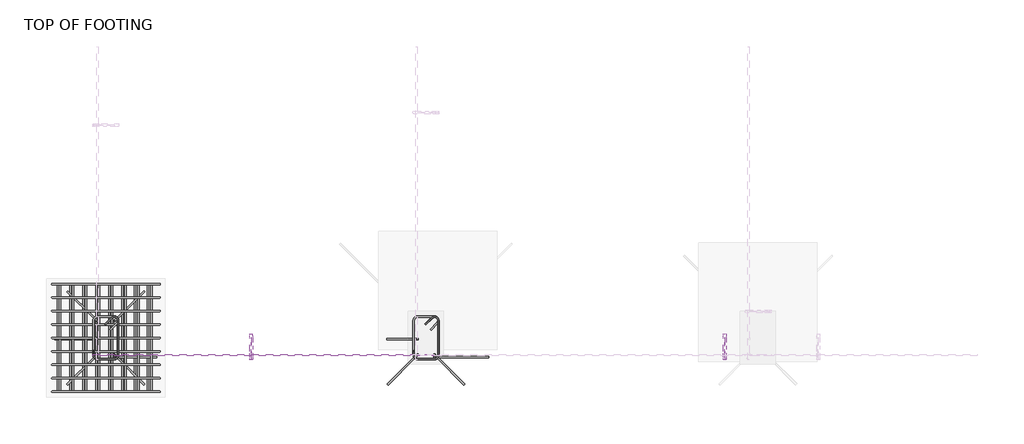
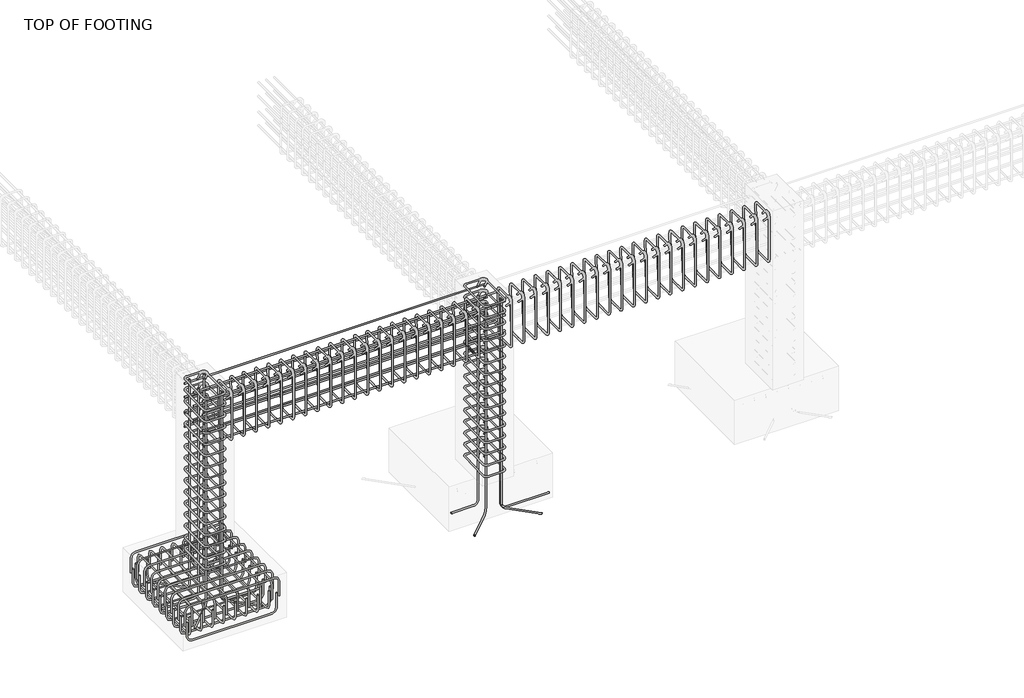
# One storey, part 2 of 14: 22 reinforcing bars.
"""IFC4 building model written with IfcOpenShell, lengths in millimetres."""

from ifc_helpers import new_model, si_unit, point, frame, origin, place, context, project, spatial, polyline, circle_curve, trimmed, segment, composite_curve, source, transform, mapped, element, save
from ifc_brep_helpers import swept_disk

model = new_model("IFC4")

# Units and contexts
model_context = context("Model", 3, world=origin())
ifc_project = project(units=[si_unit("LENGTHUNIT", "METRE", prefix="MILLI")], contexts=[model_context])

# Site, building, storey
site = spatial("IfcSite", under=ifc_project)
building = spatial("IfcBuilding", under=site)
storey = spatial("IfcBuildingStorey", under=building, Name="TOP OF FOOTING", Elevation=-1828.8)

# Reinforcing bars
placement = place(None, origin())
reinforcing_bar_shape = source(origin(), model_context, "Body", "SolidModel", [
    swept_disk(composite_curve([segment(polyline([(-3027.457813, 117.7803241, -2035.6107622), (-3027.457813, 117.7803241, -2182.9107622)]), True, "CONTINUOUS"), segment(trimmed(circle_curve(frame((-3073.807813, 117.7803241, -2182.9107622), z_axis=(0.0, 1.0, 0.0), x_axis=(46.34999999999991, 0.0, 0.0)), 46.35), [point((-3027.457813, 117.7803241, -2182.9107622))], [point((-3073.807813, 117.7803241, -2229.2607622))], True, "CARTESIAN"), True, "CONTINUOUS"), segment(polyline([(-3073.807813, 117.7803241, -2229.2607622), (-3846.4382016, 117.7803241, -2229.2607622)]), True, "CONTINUOUS"), segment(trimmed(circle_curve(frame((-3846.4382016, 117.7803241, -2182.9107622), z_axis=(0.0, 1.0, 0.0), x_axis=(0.0, 0.0, -46.34999999999991)), 46.35), [point((-3846.4382016, 117.7803241, -2229.2607622))], [point((-3892.7882016, 117.7803241, -2182.9107622))], True, "CARTESIAN"), True, "CONTINUOUS"), segment(polyline([(-3892.7882016, 117.7803241, -2182.9107622), (-3892.7882016, 117.7803241, -2035.6107622)]), True, "CONTINUOUS")], self_intersect=False), 6.35),
])
element("IfcReinforcingBar", 1, at=placement, inside=storey, context=model_context, shape_type="MappedRepresentation", body=[
    mapped(reinforcing_bar_shape, transform((0.0, 0.0, 0.0), x_axis=(1.0, 0.0, 0.0), y_axis=(0.0, 1.0, 0.0), z_axis=(0.0, 0.0, 1.0))),
    mapped(reinforcing_bar_shape, transform((0.0, -113.4125, 0.0), x_axis=(1.0, 0.0, 0.0), y_axis=(0.0, 1.0, 0.0), z_axis=(0.0, 0.0, 1.0))),
    mapped(reinforcing_bar_shape, transform((0.0, -226.825, 0.0), x_axis=(1.0, 0.0, 0.0), y_axis=(0.0, 1.0, 0.0), z_axis=(0.0, 0.0, 1.0))),
    mapped(reinforcing_bar_shape, transform((0.0, -340.2375, 0.0), x_axis=(1.0, 0.0, 0.0), y_axis=(0.0, 1.0, 0.0), z_axis=(0.0, 0.0, 1.0))),
    mapped(reinforcing_bar_shape, transform((0.0, -453.65, 0.0), x_axis=(1.0, 0.0, 0.0), y_axis=(0.0, 1.0, 0.0), z_axis=(0.0, 0.0, 1.0))),
    mapped(reinforcing_bar_shape, transform((0.0, -567.0625, 0.0), x_axis=(1.0, 0.0, 0.0), y_axis=(0.0, 1.0, 0.0), z_axis=(0.0, 0.0, 1.0))),
    mapped(reinforcing_bar_shape, transform((0.0, -680.475, 0.0), x_axis=(1.0, 0.0, 0.0), y_axis=(0.0, 1.0, 0.0), z_axis=(0.0, 0.0, 1.0))),
    mapped(reinforcing_bar_shape, transform((0.0, -793.8875, 0.0), x_axis=(1.0, 0.0, 0.0), y_axis=(0.0, 1.0, 0.0), z_axis=(0.0, 0.0, 1.0))),
    mapped(reinforcing_bar_shape, transform((0.0, -907.3, 0.0), x_axis=(1.0, 0.0, 0.0), y_axis=(0.0, 1.0, 0.0), z_axis=(0.0, 0.0, 1.0))),
])
reinforcing_bar_2_shape = source(origin(), model_context, "Body", "SolidModel", [
    swept_disk(composite_curve([segment(polyline([(-3911.0033787, 117.7803241, -2068.991024), (-3911.0033787, 117.7803241, -1921.691024)]), True, "CONTINUOUS"), segment(trimmed(circle_curve(frame((-3864.6533787, 117.7803241, -1921.691024), z_axis=(0.0, 1.0, 0.0), x_axis=(-46.350000000000364, 0.0, 0.0)), 46.35), [point((-3911.0033787, 117.7803241, -1921.691024))], [point((-3864.6533787, 117.7803241, -1875.341024))], True, "CARTESIAN"), True, "CONTINUOUS"), segment(polyline([(-3864.6533787, 117.7803241, -1875.341024), (-3050.0533787, 117.7803241, -1875.341024)]), True, "CONTINUOUS"), segment(trimmed(circle_curve(frame((-3050.0533787, 117.7803241, -1921.691024), z_axis=(0.0, 1.0, 0.0), x_axis=(0.0, 0.0, 46.34999999999991)), 46.35), [point((-3050.0533787, 117.7803241, -1875.341024))], [point((-3003.7033787, 117.7803241, -1921.691024))], True, "CARTESIAN"), True, "CONTINUOUS"), segment(polyline([(-3003.7033787, 117.7803241, -1921.691024), (-3003.7033787, 117.7803241, -2068.991024)]), True, "CONTINUOUS")], self_intersect=False), 6.35),
])
element("IfcReinforcingBar", 2, at=placement, inside=storey, context=model_context, shape_type="MappedRepresentation", body=[
    mapped(reinforcing_bar_2_shape, transform((0.0, 0.0, 0.0), x_axis=(1.0, 0.0, 0.0), y_axis=(0.0, 1.0, 0.0), z_axis=(0.0, 0.0, 1.0))),
    mapped(reinforcing_bar_2_shape, transform((0.0, -113.4125, 0.0), x_axis=(1.0, 0.0, 0.0), y_axis=(0.0, 1.0, 0.0), z_axis=(0.0, 0.0, 1.0))),
    mapped(reinforcing_bar_2_shape, transform((0.0, -226.825, 0.0), x_axis=(1.0, 0.0, 0.0), y_axis=(0.0, 1.0, 0.0), z_axis=(0.0, 0.0, 1.0))),
    mapped(reinforcing_bar_2_shape, transform((0.0, -340.2375, 0.0), x_axis=(1.0, 0.0, 0.0), y_axis=(0.0, 1.0, 0.0), z_axis=(0.0, 0.0, 1.0))),
    mapped(reinforcing_bar_2_shape, transform((0.0, -453.65, 0.0), x_axis=(1.0, 0.0, 0.0), y_axis=(0.0, 1.0, 0.0), z_axis=(0.0, 0.0, 1.0))),
    mapped(reinforcing_bar_2_shape, transform((0.0, -567.0625, 0.0), x_axis=(1.0, 0.0, 0.0), y_axis=(0.0, 1.0, 0.0), z_axis=(0.0, 0.0, 1.0))),
    mapped(reinforcing_bar_2_shape, transform((0.0, -680.475, 0.0), x_axis=(1.0, 0.0, 0.0), y_axis=(0.0, 1.0, 0.0), z_axis=(0.0, 0.0, 1.0))),
    mapped(reinforcing_bar_2_shape, transform((0.0, -793.8875, 0.0), x_axis=(1.0, 0.0, 0.0), y_axis=(0.0, 1.0, 0.0), z_axis=(0.0, 0.0, 1.0))),
    mapped(reinforcing_bar_2_shape, transform((0.0, -907.3, 0.0), x_axis=(1.0, 0.0, 0.0), y_axis=(0.0, 1.0, 0.0), z_axis=(0.0, 0.0, 1.0))),
])
reinforcing_bar_3_shape = source(origin(), model_context, "Body", "SolidModel", [
    swept_disk(composite_curve([segment(polyline([(-3073.4932847, 117.7803241, -2085.4684936), (-3073.4932847, 117.7803241, -1938.1684936)]), True, "CONTINUOUS"), segment(trimmed(circle_curve(frame((-3073.4932847, 71.4303241, -1938.1684936), z_axis=(1.0, 0.0, 0.0), x_axis=(0.0, 46.349999999999994, 0.0)), 46.35), [point((-3073.4932847, 117.7803241, -1938.1684936))], [point((-3073.4932847, 71.4303241, -1891.8184936))], True, "CARTESIAN"), True, "CONTINUOUS"), segment(polyline([(-3073.4932847, 71.4303241, -1891.8184936), (-3073.4932847, -743.1696759, -1891.8184936)]), True, "CONTINUOUS"), segment(trimmed(circle_curve(frame((-3073.4932847, -743.1696759, -1938.1684936), z_axis=(1.0, 0.0, 0.0), x_axis=(0.0, 0.0, 46.34999999999991)), 46.35), [point((-3073.4932847, -743.1696759, -1891.8184936))], [point((-3073.4932847, -789.5196759, -1938.1684936))], True, "CARTESIAN"), True, "CONTINUOUS"), segment(polyline([(-3073.4932847, -789.5196759, -1938.1684936), (-3073.4932847, -789.5196759, -2085.4684936)]), True, "CONTINUOUS")], self_intersect=False), 6.35),
])
element("IfcReinforcingBar", 3, at=placement, inside=storey, context=model_context, shape_type="MappedRepresentation", body=[
    mapped(reinforcing_bar_3_shape, transform((0.0, 0.0, 0.0), x_axis=(1.0, 0.0, 0.0), y_axis=(0.0, 1.0, 0.0), z_axis=(0.0, 0.0, 1.0))),
    mapped(reinforcing_bar_3_shape, transform((-110.0713853, 0.0, 0.0), x_axis=(1.0, 0.0, 0.0), y_axis=(0.0, 1.0, 0.0), z_axis=(0.0, 0.0, 1.0))),
    mapped(reinforcing_bar_3_shape, transform((-220.1427706, 0.0, 0.0), x_axis=(1.0, 0.0, 0.0), y_axis=(0.0, 1.0, 0.0), z_axis=(0.0, 0.0, 1.0))),
    mapped(reinforcing_bar_3_shape, transform((-330.2141558, 0.0, 0.0), x_axis=(1.0, 0.0, 0.0), y_axis=(0.0, 1.0, 0.0), z_axis=(0.0, 0.0, 1.0))),
    mapped(reinforcing_bar_3_shape, transform((-440.2855411, 0.0, 0.0), x_axis=(1.0, 0.0, 0.0), y_axis=(0.0, 1.0, 0.0), z_axis=(0.0, 0.0, 1.0))),
    mapped(reinforcing_bar_3_shape, transform((-550.3569264, 0.0, 0.0), x_axis=(1.0, 0.0, 0.0), y_axis=(0.0, 1.0, 0.0), z_axis=(0.0, 0.0, 1.0))),
    mapped(reinforcing_bar_3_shape, transform((-660.4283117, 0.0, 0.0), x_axis=(1.0, 0.0, 0.0), y_axis=(0.0, 1.0, 0.0), z_axis=(0.0, 0.0, 1.0))),
    mapped(reinforcing_bar_3_shape, transform((-770.4996969, 0.0, 0.0), x_axis=(1.0, 0.0, 0.0), y_axis=(0.0, 1.0, 0.0), z_axis=(0.0, 0.0, 1.0))),
])
reinforcing_bar_4_shape = source(origin(), model_context, "Body", "SolidModel", [
    swept_disk(composite_curve([segment(polyline([(-3862.3533787, 117.7803241, -1990.15), (-3862.3533787, 117.7803241, -2137.45)]), True, "CONTINUOUS"), segment(trimmed(circle_curve(frame((-3862.3533787, 71.4303241, -2137.45), z_axis=(-1.0, 0.0, 0.0), x_axis=(0.0, 46.349999999999994, 0.0)), 46.35), [point((-3862.3533787, 117.7803241, -2137.45))], [point((-3862.3533787, 71.4303241, -2183.8))], True, "CARTESIAN"), True, "CONTINUOUS"), segment(polyline([(-3862.3533787, 71.4303241, -2183.8), (-3862.3533787, -743.1696759, -2183.8)]), True, "CONTINUOUS"), segment(trimmed(circle_curve(frame((-3862.3533787, -743.1696759, -2137.45), z_axis=(-1.0, 0.0, 0.0), x_axis=(0.0, 0.0, -46.350000000000364)), 46.35), [point((-3862.3533787, -743.1696759, -2183.8))], [point((-3862.3533787, -789.5196759, -2137.45))], True, "CARTESIAN"), True, "CONTINUOUS"), segment(polyline([(-3862.3533787, -789.5196759, -2137.45), (-3862.3533787, -789.5196759, -1990.15)]), True, "CONTINUOUS")], self_intersect=False), 6.35),
])
element("IfcReinforcingBar", 4, at=placement, inside=storey, context=model_context, shape_type="MappedRepresentation", body=[
    mapped(reinforcing_bar_4_shape, transform((0.0, 0.0, 0.0), x_axis=(1.0, 0.0, 0.0), y_axis=(0.0, 1.0, 0.0), z_axis=(0.0, 0.0, 1.0))),
    mapped(reinforcing_bar_4_shape, transform((108.7810905, 0.0, 0.0), x_axis=(1.0, 0.0, 0.0), y_axis=(0.0, 1.0, 0.0), z_axis=(0.0, 0.0, 1.0))),
    mapped(reinforcing_bar_4_shape, transform((217.5621811, 0.0, 0.0), x_axis=(1.0, 0.0, 0.0), y_axis=(0.0, 1.0, 0.0), z_axis=(0.0, 0.0, 1.0))),
    mapped(reinforcing_bar_4_shape, transform((326.3432716, 0.0, 0.0), x_axis=(1.0, 0.0, 0.0), y_axis=(0.0, 1.0, 0.0), z_axis=(0.0, 0.0, 1.0))),
    mapped(reinforcing_bar_4_shape, transform((435.1243621, 0.0, 0.0), x_axis=(1.0, 0.0, 0.0), y_axis=(0.0, 1.0, 0.0), z_axis=(0.0, 0.0, 1.0))),
    mapped(reinforcing_bar_4_shape, transform((543.9054526, 0.0, 0.0), x_axis=(1.0, 0.0, 0.0), y_axis=(0.0, 1.0, 0.0), z_axis=(0.0, 0.0, 1.0))),
    mapped(reinforcing_bar_4_shape, transform((652.6865432, 0.0, 0.0), x_axis=(1.0, 0.0, 0.0), y_axis=(0.0, 1.0, 0.0), z_axis=(0.0, 0.0, 1.0))),
    mapped(reinforcing_bar_4_shape, transform((761.4676337, 0.0, 0.0), x_axis=(1.0, 0.0, 0.0), y_axis=(0.0, 1.0, 0.0), z_axis=(0.0, 0.0, 1.0))),
])
reinforcing_bar_5_shape = source(origin(), model_context, "Body", "SolidModel", [
    swept_disk(composite_curve([segment(polyline([(-3462.9647392, -222.1454413, -46.35), (-3407.2211763, -166.4018783, -46.35)]), True, "CONTINUOUS"), segment(trimmed(circle_curve(frame((-3385.0533787, -188.5696759, -46.35), z_axis=(0.0, 0.0, -1.0), x_axis=(-22.167797600000085, 22.1677976, 0.0)), 31.35), [point((-3407.2211763, -166.4018783, -46.35))], [point((-3353.7033787, -188.5696759, -46.35))], True, "CARTESIAN"), True, "CONTINUOUS"), segment(polyline([(-3353.7033787, -188.5696759, -46.35), (-3353.7033787, -483.1696759, -46.35)]), True, "CONTINUOUS"), segment(trimmed(circle_curve(frame((-3385.0533787, -483.1696759, -46.35), z_axis=(0.0, 0.0, -1.0), x_axis=(31.34999999999991, 0.0, 0.0)), 31.35), [point((-3353.7033787, -483.1696759, -46.35))], [point((-3385.0533787, -514.5196759, -46.35))], True, "CARTESIAN"), True, "CONTINUOUS"), segment(polyline([(-3385.0533787, -514.5196759, -46.35), (-3529.6533787, -514.5196759, -46.35)]), True, "CONTINUOUS"), segment(trimmed(circle_curve(frame((-3529.6533787, -483.189461, -45.2363875), z_axis=(0.0, 0.03552192833448213, -0.9993688971583016), x_axis=(0.0, -31.330214900000044, -1.1136125000000021)), 31.35), [point((-3529.6533787, -514.5196759, -46.35))], [point((-3561.0033787, -483.189461, -45.2363875))], True, "CARTESIAN"), True, "CONTINUOUS"), segment(polyline([(-3561.0033787, -483.189461, -45.2363875), (-3561.0033787, -188.5498908, -34.7636125)]), True, "CONTINUOUS"), segment(trimmed(circle_curve(frame((-3529.6533787, -188.5498908, -34.7636125), z_axis=(0.0, 0.03552192833448213, -0.9993688971583016), x_axis=(-31.350000000000364, 0.0, 0.0)), 31.35), [point((-3561.0033787, -188.5498908, -34.7636125))], [point((-3529.6533787, -157.2196759, -33.65))], True, "CARTESIAN"), True, "CONTINUOUS"), segment(polyline([(-3529.6533787, -157.2196759, -33.65), (-3385.0533787, -157.2196759, -33.65)]), True, "CONTINUOUS"), segment(trimmed(circle_curve(frame((-3385.0533787, -188.5696759, -33.65), z_axis=(0.0, 0.0, -1.0), x_axis=(0.0, 31.349999999999994, 0.0)), 31.35), [point((-3385.0533787, -157.2196759, -33.65))], [point((-3362.8855811, -210.7374735, -33.65))], True, "CARTESIAN"), True, "CONTINUOUS"), segment(polyline([(-3362.8855811, -210.7374735, -33.65), (-3418.6291441, -266.4810364, -33.65)]), True, "CONTINUOUS")], self_intersect=False), 6.35),
])
element("IfcReinforcingBar", 5, at=placement, inside=storey, context=model_context, shape_type="MappedRepresentation", body=[
    mapped(reinforcing_bar_5_shape, transform((0.0, 0.0, 0.0), x_axis=(1.0, 0.0, 0.0), y_axis=(0.0, 1.0, 0.0), z_axis=(0.0, 0.0, 1.0))),
    mapped(reinforcing_bar_5_shape, transform((0.0, 0.0, -115.74), x_axis=(1.0, 0.0, 0.0), y_axis=(0.0, 1.0, 0.0), z_axis=(0.0, 0.0, 1.0))),
    mapped(reinforcing_bar_5_shape, transform((0.0, 0.0, -231.48), x_axis=(1.0, 0.0, 0.0), y_axis=(0.0, 1.0, 0.0), z_axis=(0.0, 0.0, 1.0))),
    mapped(reinforcing_bar_5_shape, transform((0.0, 0.0, -347.22), x_axis=(1.0, 0.0, 0.0), y_axis=(0.0, 1.0, 0.0), z_axis=(0.0, 0.0, 1.0))),
    mapped(reinforcing_bar_5_shape, transform((0.0, 0.0, -462.96), x_axis=(1.0, 0.0, 0.0), y_axis=(0.0, 1.0, 0.0), z_axis=(0.0, 0.0, 1.0))),
    mapped(reinforcing_bar_5_shape, transform((0.0, 0.0, -578.7), x_axis=(1.0, 0.0, 0.0), y_axis=(0.0, 1.0, 0.0), z_axis=(0.0, 0.0, 1.0))),
    mapped(reinforcing_bar_5_shape, transform((0.0, 0.0, -694.44), x_axis=(1.0, 0.0, 0.0), y_axis=(0.0, 1.0, 0.0), z_axis=(0.0, 0.0, 1.0))),
    mapped(reinforcing_bar_5_shape, transform((0.0, 0.0, -810.18), x_axis=(1.0, 0.0, 0.0), y_axis=(0.0, 1.0, 0.0), z_axis=(0.0, 0.0, 1.0))),
    mapped(reinforcing_bar_5_shape, transform((0.0, 0.0, -925.92), x_axis=(1.0, 0.0, 0.0), y_axis=(0.0, 1.0, 0.0), z_axis=(0.0, 0.0, 1.0))),
    mapped(reinforcing_bar_5_shape, transform((0.0, 0.0, -1041.66), x_axis=(1.0, 0.0, 0.0), y_axis=(0.0, 1.0, 0.0), z_axis=(0.0, 0.0, 1.0))),
    mapped(reinforcing_bar_5_shape, transform((0.0, 0.0, -1157.4), x_axis=(1.0, 0.0, 0.0), y_axis=(0.0, 1.0, 0.0), z_axis=(0.0, 0.0, 1.0))),
    mapped(reinforcing_bar_5_shape, transform((0.0, 0.0, -1273.14), x_axis=(1.0, 0.0, 0.0), y_axis=(0.0, 1.0, 0.0), z_axis=(0.0, 0.0, 1.0))),
    mapped(reinforcing_bar_5_shape, transform((0.0, 0.0, -1388.88), x_axis=(1.0, 0.0, 0.0), y_axis=(0.0, 1.0, 0.0), z_axis=(0.0, 0.0, 1.0))),
    mapped(reinforcing_bar_5_shape, transform((0.0, 0.0, -1504.62), x_axis=(1.0, 0.0, 0.0), y_axis=(0.0, 1.0, 0.0), z_axis=(0.0, 0.0, 1.0))),
    mapped(reinforcing_bar_5_shape, transform((0.0, 0.0, -1620.36), x_axis=(1.0, 0.0, 0.0), y_axis=(0.0, 1.0, 0.0), z_axis=(0.0, 0.0, 1.0))),
    mapped(reinforcing_bar_5_shape, transform((0.0, 0.0, -1736.1), x_axis=(1.0, 0.0, 0.0), y_axis=(0.0, 1.0, 0.0), z_axis=(0.0, 0.0, 1.0))),
])
element("IfcReinforcingBar", 6, at=placement, inside=storey, context=model_context, shape_type="SolidModel", body=[
    swept_disk(composite_curve([segment(polyline([(-3386.7020371, -495.9487744, -40.0), (-3386.7020371, -495.9487744, -2122.4113862)]), True, "CONTINUOUS"), segment(trimmed(circle_curve(frame((-3340.3520371, -495.9487744, -2122.4113862), z_axis=(0.0, -1.0, 0.0), x_axis=(-46.34999999999991, 0.0, 0.0)), 46.35), [point((-3386.7020371, -495.9487744, -2122.4113862))], [point((-3340.3520371, -495.9487744, -2168.7613862))], True, "CARTESIAN"), True, "CONTINUOUS"), segment(polyline([(-3340.3520371, -495.9487744, -2168.7613862), (-3028.2406023, -495.9487744, -2168.7613862)]), True, "CONTINUOUS")], self_intersect=False), 6.35),
])
element("IfcReinforcingBar", 7, at=placement, inside=storey, context=model_context, shape_type="SolidModel", body=[
    swept_disk(composite_curve([segment(polyline([(-3386.7020371, -475.9487744, -40.0), (-3386.7020371, -475.9487744, -2122.4113862)]), True, "CONTINUOUS"), segment(trimmed(circle_curve(frame((-3353.9276378, -508.7231737, -2122.4113862), z_axis=(-0.7071067811865441, -0.707106781186551, 0.0), x_axis=(-32.774399299999914, 32.77439930000003, 0.0)), 46.35), [point((-3386.7020371, -475.9487744, -2122.4113862))], [point((-3353.9276378, -508.7231737, -2168.7613862))], True, "CARTESIAN"), True, "CONTINUOUS"), segment(polyline([(-3353.9276378, -508.7231737, -2168.7613862), (-3133.2315258, -729.4192858, -2168.7613862)]), True, "CONTINUOUS")], self_intersect=False), 6.35),
])
element("IfcReinforcingBar", 8, at=placement, inside=storey, context=model_context, shape_type="SolidModel", body=[
    swept_disk(composite_curve([segment(polyline([(-3528.0047203, -475.9487744, -40.0), (-3528.0047203, -475.9487744, -2122.4113862)]), True, "CONTINUOUS"), segment(trimmed(circle_curve(frame((-3560.7791196, -508.7231737, -2122.4113862), z_axis=(-0.7071067811865341, 0.707106781186561, 0.0), x_axis=(32.774399299999914, 32.77439930000003, 0.0)), 46.35), [point((-3528.0047203, -475.9487744, -2122.4113862))], [point((-3560.7791196, -508.7231737, -2168.7613862))], True, "CARTESIAN"), True, "CONTINUOUS"), segment(polyline([(-3560.7791196, -508.7231737, -2168.7613862), (-3781.4752316, -729.4192858, -2168.7613862)]), True, "CONTINUOUS")], self_intersect=False), 6.35),
])
element("IfcReinforcingBar", 9, at=placement, inside=storey, context=model_context, shape_type="SolidModel", body=[
    swept_disk(composite_curve([segment(polyline([(-3386.7020371, -195.7905774, -40.0), (-3386.7020371, -195.7905774, -2122.4113862)]), True, "CONTINUOUS"), segment(trimmed(circle_curve(frame((-3353.9276378, -163.0161781, -2122.4113862), z_axis=(0.7071067811865235, -0.7071067811865717, 0.0), x_axis=(-32.774399299999914, -32.7743993, 0.0)), 46.35), [point((-3386.7020371, -195.7905774, -2122.4113862))], [point((-3353.9276378, -163.0161781, -2168.7613862))], True, "CARTESIAN"), True, "CONTINUOUS"), segment(polyline([(-3353.9276378, -163.0161781, -2168.7613862), (-3133.2315258, 57.6799339, -2168.7613862)]), True, "CONTINUOUS")], self_intersect=False), 6.35),
])
element("IfcReinforcingBar", 10, at=placement, inside=storey, context=model_context, shape_type="SolidModel", body=[
    swept_disk(composite_curve([segment(polyline([(-3528.0047203, -195.7905774, -40.0), (-3528.0047203, -195.7905774, -2122.4113862)]), True, "CONTINUOUS"), segment(trimmed(circle_curve(frame((-3560.7791196, -163.0161781, -2122.4113862), z_axis=(0.7071067811865548, 0.7071067811865404, 0.0), x_axis=(32.774399299999914, -32.7743993, 0.0)), 46.35), [point((-3528.0047203, -195.7905774, -2122.4113862))], [point((-3560.7791196, -163.0161781, -2168.7613862))], True, "CARTESIAN"), True, "CONTINUOUS"), segment(polyline([(-3560.7791196, -163.0161781, -2168.7613862), (-3781.4752316, 57.6799339, -2168.7613862)]), True, "CONTINUOUS")], self_intersect=False), 6.35),
])
element("IfcReinforcingBar", 11, at=placement, inside=storey, context=model_context, shape_type="SolidModel", body=[
    swept_disk(composite_curve([segment(polyline([(-3528.0047203, -345.9487744, -40.0), (-3528.0047203, -345.9487744, -2122.4113862)]), True, "CONTINUOUS"), segment(trimmed(circle_curve(frame((-3574.3547203, -345.9487744, -2122.4113862), z_axis=(0.0, 1.0, 0.0), x_axis=(46.34999999999991, 0.0, 0.0)), 46.35), [point((-3528.0047203, -345.9487744, -2122.4113862))], [point((-3574.3547203, -345.9487744, -2168.7613862))], True, "CARTESIAN"), True, "CONTINUOUS"), segment(polyline([(-3574.3547203, -345.9487744, -2168.7613862), (-3886.4661551, -345.9487744, -2168.7613862)]), True, "CONTINUOUS")], self_intersect=False), 6.35),
])
reinforcing_bar_6_shape = source(origin(), model_context, "Body", "SolidModel", [
    swept_disk(composite_curve([segment(polyline([(-762.9647392, -222.1454413, -46.35), (-707.2211763, -166.4018783, -46.35)]), True, "CONTINUOUS"), segment(trimmed(circle_curve(frame((-685.0533787, -188.5696759, -46.35), z_axis=(0.0, 0.0, -1.0), x_axis=(-22.16779759999997, 22.1677976, 0.0)), 31.35), [point((-707.2211763, -166.4018783, -46.35))], [point((-653.7033787, -188.5696759, -46.35))], True, "CARTESIAN"), True, "CONTINUOUS"), segment(polyline([(-653.7033787, -188.5696759, -46.35), (-653.7033787, -483.1696759, -46.35)]), True, "CONTINUOUS"), segment(trimmed(circle_curve(frame((-685.0533787, -483.1696759, -46.35), z_axis=(0.0, 0.0, -1.0), x_axis=(31.350000000000023, 0.0, 0.0)), 31.35), [point((-653.7033787, -483.1696759, -46.35))], [point((-685.0533787, -514.5196759, -46.35))], True, "CARTESIAN"), True, "CONTINUOUS"), segment(polyline([(-685.0533787, -514.5196759, -46.35), (-829.6533787, -514.5196759, -46.35)]), True, "CONTINUOUS"), segment(trimmed(circle_curve(frame((-829.6533787, -483.189461, -45.2363875), z_axis=(0.0, 0.03552192833448213, -0.9993688971583016), x_axis=(0.0, -31.330214900000044, -1.1136125000000021)), 31.35), [point((-829.6533787, -514.5196759, -46.35))], [point((-861.0033787, -483.189461, -45.2363875))], True, "CARTESIAN"), True, "CONTINUOUS"), segment(polyline([(-861.0033787, -483.189461, -45.2363875), (-861.0033787, -188.5498908, -34.7636125)]), True, "CONTINUOUS"), segment(trimmed(circle_curve(frame((-829.6533787, -188.5498908, -34.7636125), z_axis=(0.0, 0.03552192833448213, -0.9993688971583016), x_axis=(-31.350000000000023, 0.0, 0.0)), 31.35), [point((-861.0033787, -188.5498908, -34.7636125))], [point((-829.6533787, -157.2196759, -33.65))], True, "CARTESIAN"), True, "CONTINUOUS"), segment(polyline([(-829.6533787, -157.2196759, -33.65), (-685.0533787, -157.2196759, -33.65)]), True, "CONTINUOUS"), segment(trimmed(circle_curve(frame((-685.0533787, -188.5696759, -33.65), z_axis=(0.0, 0.0, -1.0), x_axis=(0.0, 31.349999999999994, 0.0)), 31.35), [point((-685.0533787, -157.2196759, -33.65))], [point((-662.8855811, -210.7374735, -33.65))], True, "CARTESIAN"), True, "CONTINUOUS"), segment(polyline([(-662.8855811, -210.7374735, -33.65), (-718.6291441, -266.4810364, -33.65)]), True, "CONTINUOUS")], self_intersect=False), 6.35),
])
element("IfcReinforcingBar", 12, at=placement, inside=storey, context=model_context, shape_type="MappedRepresentation", body=[
    mapped(reinforcing_bar_6_shape, transform((0.0, 0.0, 0.0), x_axis=(1.0, 0.0, 0.0), y_axis=(0.0, 1.0, 0.0), z_axis=(0.0, 0.0, 1.0))),
    mapped(reinforcing_bar_6_shape, transform((0.0, 0.0, -115.74), x_axis=(1.0, 0.0, 0.0), y_axis=(0.0, 1.0, 0.0), z_axis=(0.0, 0.0, 1.0))),
    mapped(reinforcing_bar_6_shape, transform((0.0, 0.0, -231.48), x_axis=(1.0, 0.0, 0.0), y_axis=(0.0, 1.0, 0.0), z_axis=(0.0, 0.0, 1.0))),
    mapped(reinforcing_bar_6_shape, transform((0.0, 0.0, -347.22), x_axis=(1.0, 0.0, 0.0), y_axis=(0.0, 1.0, 0.0), z_axis=(0.0, 0.0, 1.0))),
    mapped(reinforcing_bar_6_shape, transform((0.0, 0.0, -462.96), x_axis=(1.0, 0.0, 0.0), y_axis=(0.0, 1.0, 0.0), z_axis=(0.0, 0.0, 1.0))),
    mapped(reinforcing_bar_6_shape, transform((0.0, 0.0, -578.7), x_axis=(1.0, 0.0, 0.0), y_axis=(0.0, 1.0, 0.0), z_axis=(0.0, 0.0, 1.0))),
    mapped(reinforcing_bar_6_shape, transform((0.0, 0.0, -694.44), x_axis=(1.0, 0.0, 0.0), y_axis=(0.0, 1.0, 0.0), z_axis=(0.0, 0.0, 1.0))),
    mapped(reinforcing_bar_6_shape, transform((0.0, 0.0, -810.18), x_axis=(1.0, 0.0, 0.0), y_axis=(0.0, 1.0, 0.0), z_axis=(0.0, 0.0, 1.0))),
    mapped(reinforcing_bar_6_shape, transform((0.0, 0.0, -925.92), x_axis=(1.0, 0.0, 0.0), y_axis=(0.0, 1.0, 0.0), z_axis=(0.0, 0.0, 1.0))),
    mapped(reinforcing_bar_6_shape, transform((0.0, 0.0, -1041.66), x_axis=(1.0, 0.0, 0.0), y_axis=(0.0, 1.0, 0.0), z_axis=(0.0, 0.0, 1.0))),
    mapped(reinforcing_bar_6_shape, transform((0.0, 0.0, -1157.4), x_axis=(1.0, 0.0, 0.0), y_axis=(0.0, 1.0, 0.0), z_axis=(0.0, 0.0, 1.0))),
    mapped(reinforcing_bar_6_shape, transform((0.0, 0.0, -1273.14), x_axis=(1.0, 0.0, 0.0), y_axis=(0.0, 1.0, 0.0), z_axis=(0.0, 0.0, 1.0))),
    mapped(reinforcing_bar_6_shape, transform((0.0, 0.0, -1388.88), x_axis=(1.0, 0.0, 0.0), y_axis=(0.0, 1.0, 0.0), z_axis=(0.0, 0.0, 1.0))),
    mapped(reinforcing_bar_6_shape, transform((0.0, 0.0, -1504.62), x_axis=(1.0, 0.0, 0.0), y_axis=(0.0, 1.0, 0.0), z_axis=(0.0, 0.0, 1.0))),
    mapped(reinforcing_bar_6_shape, transform((0.0, 0.0, -1620.36), x_axis=(1.0, 0.0, 0.0), y_axis=(0.0, 1.0, 0.0), z_axis=(0.0, 0.0, 1.0))),
    mapped(reinforcing_bar_6_shape, transform((0.0, 0.0, -1736.1), x_axis=(1.0, 0.0, 0.0), y_axis=(0.0, 1.0, 0.0), z_axis=(0.0, 0.0, 1.0))),
])
element("IfcReinforcingBar", 13, at=placement, inside=storey, context=model_context, shape_type="SolidModel", body=[
    swept_disk(composite_curve([segment(polyline([(-686.7020371, -495.9487744, -40.0), (-686.7020371, -495.9487744, -2122.4113862)]), True, "CONTINUOUS"), segment(trimmed(circle_curve(frame((-640.3520371, -495.9487744, -2122.4113862), z_axis=(0.0, -1.0, 0.0), x_axis=(-46.35000000000002, 0.0, 0.0)), 46.35), [point((-686.7020371, -495.9487744, -2122.4113862))], [point((-640.3520371, -495.9487744, -2168.7613862))], True, "CARTESIAN"), True, "CONTINUOUS"), segment(polyline([(-640.3520371, -495.9487744, -2168.7613862), (-228.2406023, -495.9487744, -2168.7613862)]), True, "CONTINUOUS")], self_intersect=False), 6.35),
])
element("IfcReinforcingBar", 14, at=placement, inside=storey, context=model_context, shape_type="SolidModel", body=[
    swept_disk(composite_curve([segment(polyline([(-686.7020371, -475.9487744, -40.0), (-686.7020371, -475.9487744, -2122.4113862)]), True, "CONTINUOUS"), segment(trimmed(circle_curve(frame((-653.9276378, -508.7231737, -2122.4113862), z_axis=(-0.7071067811865441, -0.707106781186551, 0.0), x_axis=(-32.77439930000003, 32.77439930000003, 0.0)), 46.35), [point((-686.7020371, -475.9487744, -2122.4113862))], [point((-653.9276378, -508.7231737, -2168.7613862))], True, "CARTESIAN"), True, "CONTINUOUS"), segment(polyline([(-653.9276378, -508.7231737, -2168.7613862), (-433.2315258, -729.4192858, -2168.7613862)]), True, "CONTINUOUS")], self_intersect=False), 6.35),
])
element("IfcReinforcingBar", 15, at=placement, inside=storey, context=model_context, shape_type="SolidModel", body=[
    swept_disk(composite_curve([segment(polyline([(-828.0047203, -475.9487744, -40.0), (-828.0047203, -475.9487744, -2122.4113862)]), True, "CONTINUOUS"), segment(trimmed(circle_curve(frame((-860.7791196, -508.7231737, -2122.4113862), z_axis=(-0.7071067811865341, 0.707106781186561, 0.0), x_axis=(32.774399299999914, 32.77439930000003, 0.0)), 46.35), [point((-828.0047203, -475.9487744, -2122.4113862))], [point((-860.7791196, -508.7231737, -2168.7613862))], True, "CARTESIAN"), True, "CONTINUOUS"), segment(polyline([(-860.7791196, -508.7231737, -2168.7613862), (-1081.4752316, -729.4192858, -2168.7613862)]), True, "CONTINUOUS")], self_intersect=False), 6.35),
])
element("IfcReinforcingBar", 16, at=placement, inside=storey, context=model_context, shape_type="SolidModel", body=[
    swept_disk(composite_curve([segment(polyline([(-828.0047203, -345.9487744, -40.0), (-828.0047203, -345.9487744, -2122.4113862)]), True, "CONTINUOUS"), segment(trimmed(circle_curve(frame((-874.3547203, -345.9487744, -2122.4113862), z_axis=(0.0, 1.0, 0.0), x_axis=(46.35000000000002, 0.0, 0.0)), 46.35), [point((-828.0047203, -345.9487744, -2122.4113862))], [point((-874.3547203, -345.9487744, -2168.7613862))], True, "CARTESIAN"), True, "CONTINUOUS"), segment(polyline([(-874.3547203, -345.9487744, -2168.7613862), (-1086.4661551, -345.9487744, -2168.7613862)]), True, "CONTINUOUS")], self_intersect=False), 6.35),
])
reinforcing_bar_7_shape = source(origin(), model_context, "Body", "SolidModel", [
    swept_disk(composite_curve([segment(polyline([(-3301.0033793, -405.2583154, -111.2757654), (-3301.0033793, -461.0018783, -55.5322024)]), True, "CONTINUOUS"), segment(trimmed(circle_curve(frame((-3301.0033793, -483.1696759, -77.7), z_axis=(1.0, 0.0, 0.0), x_axis=(0.0, 22.16779760000003, 22.1677976)), 31.35), [point((-3301.0033793, -461.0018783, -55.5322024))], [point((-3301.0033793, -514.5196759, -77.7))], True, "CARTESIAN"), True, "CONTINUOUS"), segment(polyline([(-3301.0033793, -514.5196759, -77.7), (-3301.0033793, -514.5196759, -522.3)]), True, "CONTINUOUS"), segment(trimmed(circle_curve(frame((-3301.0033793, -483.1696759, -522.3), z_axis=(1.0, 0.0, 0.0), x_axis=(0.0, -31.350000000000023, 0.0)), 31.35), [point((-3301.0033793, -514.5196759, -522.3))], [point((-3301.0033793, -483.1696759, -553.65))], True, "CARTESIAN"), True, "CONTINUOUS"), segment(polyline([(-3301.0033793, -483.1696759, -553.65), (-3301.0033793, -338.5696759, -553.65)]), True, "CONTINUOUS"), segment(trimmed(circle_curve(frame((-3301.787965, -338.5696759, -522.3098193), z_axis=(0.9996867842138424, 0.0, 0.025026655153786322), x_axis=(0.784585700000207, 0.0, -31.34018070000002)), 31.35), [point((-3301.0033793, -338.5696759, -553.65))], [point((-3301.787965, -307.2196759, -522.3098193))], True, "CARTESIAN"), True, "CONTINUOUS"), segment(polyline([(-3301.787965, -307.2196759, -522.3098193), (-3312.9187937, -307.2196759, -77.6901807)]), True, "CONTINUOUS"), segment(trimmed(circle_curve(frame((-3312.9187937, -338.5696759, -77.6901807), z_axis=(0.9996867842138424, 0.0, 0.025026655153786322), x_axis=(0.0, 31.349999999999966, 0.0)), 31.35), [point((-3312.9187937, -307.2196759, -77.6901807))], [point((-3313.7033793, -338.5696759, -46.35))], True, "CARTESIAN"), True, "CONTINUOUS"), segment(polyline([(-3313.7033793, -338.5696759, -46.35), (-3313.7033793, -483.1696759, -46.35)]), True, "CONTINUOUS"), segment(trimmed(circle_curve(frame((-3313.7033793, -483.1696759, -77.7), z_axis=(1.0, 0.0, 0.0), x_axis=(0.0, 0.0, 31.35)), 31.35), [point((-3313.7033793, -483.1696759, -46.35))], [point((-3313.7033793, -505.3374735, -99.8677976))], True, "CARTESIAN"), True, "CONTINUOUS"), segment(polyline([(-3313.7033793, -505.3374735, -99.8677976), (-3313.7033793, -449.5939106, -155.6113605)]), True, "CONTINUOUS")], self_intersect=False), 6.35),
])
element("IfcReinforcingBar", 17, at=placement, inside=storey, context=model_context, shape_type="MappedRepresentation", body=[
    mapped(reinforcing_bar_7_shape, transform((0.0, 0.0, 0.0), x_axis=(1.0, 0.0, 0.0), y_axis=(0.0, 1.0, 0.0), z_axis=(0.0, 0.0, 1.0))),
    mapped(reinforcing_bar_7_shape, transform((119.365, 0.0, 0.0), x_axis=(1.0, 0.0, 0.0), y_axis=(0.0, 1.0, 0.0), z_axis=(0.0, 0.0, 1.0))),
    mapped(reinforcing_bar_7_shape, transform((238.7300001, 0.0, 0.0), x_axis=(1.0, 0.0, 0.0), y_axis=(0.0, 1.0, 0.0), z_axis=(0.0, 0.0, 1.0))),
    mapped(reinforcing_bar_7_shape, transform((358.0950001, 0.0, 0.0), x_axis=(1.0, 0.0, 0.0), y_axis=(0.0, 1.0, 0.0), z_axis=(0.0, 0.0, 1.0))),
    mapped(reinforcing_bar_7_shape, transform((477.4600001, 0.0, 0.0), x_axis=(1.0, 0.0, 0.0), y_axis=(0.0, 1.0, 0.0), z_axis=(0.0, 0.0, 1.0))),
    mapped(reinforcing_bar_7_shape, transform((596.8250002, 0.0, 0.0), x_axis=(1.0, 0.0, 0.0), y_axis=(0.0, 1.0, 0.0), z_axis=(0.0, 0.0, 1.0))),
    mapped(reinforcing_bar_7_shape, transform((716.1900002, 0.0, 0.0), x_axis=(1.0, 0.0, 0.0), y_axis=(0.0, 1.0, 0.0), z_axis=(0.0, 0.0, 1.0))),
    mapped(reinforcing_bar_7_shape, transform((835.5550002, 0.0, 0.0), x_axis=(1.0, 0.0, 0.0), y_axis=(0.0, 1.0, 0.0), z_axis=(0.0, 0.0, 1.0))),
    mapped(reinforcing_bar_7_shape, transform((954.9200002, 0.0, 0.0), x_axis=(1.0, 0.0, 0.0), y_axis=(0.0, 1.0, 0.0), z_axis=(0.0, 0.0, 1.0))),
    mapped(reinforcing_bar_7_shape, transform((1074.2850003, 0.0, 0.0), x_axis=(1.0, 0.0, 0.0), y_axis=(0.0, 1.0, 0.0), z_axis=(0.0, 0.0, 1.0))),
    mapped(reinforcing_bar_7_shape, transform((1193.6500003, 0.0, 0.0), x_axis=(1.0, 0.0, 0.0), y_axis=(0.0, 1.0, 0.0), z_axis=(0.0, 0.0, 1.0))),
    mapped(reinforcing_bar_7_shape, transform((1313.0150003, 0.0, 0.0), x_axis=(1.0, 0.0, 0.0), y_axis=(0.0, 1.0, 0.0), z_axis=(0.0, 0.0, 1.0))),
    mapped(reinforcing_bar_7_shape, transform((1432.3800004, 0.0, 0.0), x_axis=(1.0, 0.0, 0.0), y_axis=(0.0, 1.0, 0.0), z_axis=(0.0, 0.0, 1.0))),
    mapped(reinforcing_bar_7_shape, transform((1551.7450004, 0.0, 0.0), x_axis=(1.0, 0.0, 0.0), y_axis=(0.0, 1.0, 0.0), z_axis=(0.0, 0.0, 1.0))),
    mapped(reinforcing_bar_7_shape, transform((1671.1100004, 0.0, 0.0), x_axis=(1.0, 0.0, 0.0), y_axis=(0.0, 1.0, 0.0), z_axis=(0.0, 0.0, 1.0))),
    mapped(reinforcing_bar_7_shape, transform((1790.4750005, 0.0, 0.0), x_axis=(1.0, 0.0, 0.0), y_axis=(0.0, 1.0, 0.0), z_axis=(0.0, 0.0, 1.0))),
    mapped(reinforcing_bar_7_shape, transform((1909.8400005, 0.0, 0.0), x_axis=(1.0, 0.0, 0.0), y_axis=(0.0, 1.0, 0.0), z_axis=(0.0, 0.0, 1.0))),
    mapped(reinforcing_bar_7_shape, transform((2029.2050005, 0.0, 0.0), x_axis=(1.0, 0.0, 0.0), y_axis=(0.0, 1.0, 0.0), z_axis=(0.0, 0.0, 1.0))),
    mapped(reinforcing_bar_7_shape, transform((2148.5700005, 0.0, 0.0), x_axis=(1.0, 0.0, 0.0), y_axis=(0.0, 1.0, 0.0), z_axis=(0.0, 0.0, 1.0))),
    mapped(reinforcing_bar_7_shape, transform((2267.9350006, 0.0, 0.0), x_axis=(1.0, 0.0, 0.0), y_axis=(0.0, 1.0, 0.0), z_axis=(0.0, 0.0, 1.0))),
    mapped(reinforcing_bar_7_shape, transform((2387.3000006, 0.0, 0.0), x_axis=(1.0, 0.0, 0.0), y_axis=(0.0, 1.0, 0.0), z_axis=(0.0, 0.0, 1.0))),
])
reinforcing_bar_8_shape = source(origin(), model_context, "Body", "SolidModel", [
    swept_disk(composite_curve([segment(polyline([(-3567.3533787, -181.1234225, -77.7), (-647.3533787, -181.1234225, -77.7)]), True, "CONTINUOUS")], self_intersect=False), 6.35),
])
element("IfcReinforcingBar", 18, at=placement, inside=storey, context=model_context, shape_type="MappedRepresentation", body=[
    mapped(reinforcing_bar_8_shape, transform((0.0, 0.0, 0.0), x_axis=(1.0, 0.0, 0.0), y_axis=(0.0, 1.0, 0.0), z_axis=(0.0, 0.0, 1.0))),
    mapped(reinforcing_bar_8_shape, transform((0.0, -151.0102945, 0.0), x_axis=(1.0, 0.0, 0.0), y_axis=(0.0, 1.0, 0.0), z_axis=(0.0, 0.0, 1.0))),
    mapped(reinforcing_bar_8_shape, transform((0.0, -302.0205889, 0.0), x_axis=(1.0, 0.0, 0.0), y_axis=(0.0, 1.0, 0.0), z_axis=(0.0, 0.0, 1.0))),
])
reinforcing_bar_9_shape = source(origin(), model_context, "Body", "SolidModel", [
    swept_disk(composite_curve([segment(polyline([(-3567.3533787, -181.1234225, -517.7), (-647.3533787, -181.1234225, -517.7)]), True, "CONTINUOUS")], self_intersect=False), 6.35),
])
element("IfcReinforcingBar", 19, at=placement, inside=storey, context=model_context, shape_type="MappedRepresentation", body=[
    mapped(reinforcing_bar_9_shape, transform((0.0, 0.0, 0.0), x_axis=(1.0, 0.0, 0.0), y_axis=(0.0, 1.0, 0.0), z_axis=(0.0, 0.0, 1.0))),
    mapped(reinforcing_bar_9_shape, transform((0.0, -151.0102945, 0.0), x_axis=(1.0, 0.0, 0.0), y_axis=(0.0, 1.0, 0.0), z_axis=(0.0, 0.0, 1.0))),
    mapped(reinforcing_bar_9_shape, transform((0.0, -302.0205889, 0.0), x_axis=(1.0, 0.0, 0.0), y_axis=(0.0, 1.0, 0.0), z_axis=(0.0, 0.0, 1.0))),
])
reinforcing_bar_10_shape = source(origin(), model_context, "Body", "SolidModel", [
    swept_disk(composite_curve([segment(polyline([(-3567.3533787, -181.1234225, -377.7), (-647.3533787, -181.1234225, -377.7)]), True, "CONTINUOUS")], self_intersect=False), 6.35),
])
element("IfcReinforcingBar", 20, at=placement, inside=storey, context=model_context, shape_type="MappedRepresentation", body=[
    mapped(reinforcing_bar_10_shape, transform((0.0, 0.0, 0.0), x_axis=(1.0, 0.0, 0.0), y_axis=(0.0, 1.0, 0.0), z_axis=(0.0, 0.0, 1.0))),
    mapped(reinforcing_bar_10_shape, transform((0.0, -151.0102945, 0.0), x_axis=(1.0, 0.0, 0.0), y_axis=(0.0, 1.0, 0.0), z_axis=(0.0, 0.0, 1.0))),
    mapped(reinforcing_bar_10_shape, transform((0.0, -302.0205889, 0.0), x_axis=(1.0, 0.0, 0.0), y_axis=(0.0, 1.0, 0.0), z_axis=(0.0, 0.0, 1.0))),
])
reinforcing_bar_11_shape = source(origin(), model_context, "Body", "SolidModel", [
    swept_disk(composite_curve([segment(polyline([(-3567.3533787, -181.1234225, -217.7), (-647.3533787, -181.1234225, -217.7)]), True, "CONTINUOUS")], self_intersect=False), 6.35),
])
element("IfcReinforcingBar", 21, at=placement, inside=storey, context=model_context, shape_type="MappedRepresentation", body=[
    mapped(reinforcing_bar_11_shape, transform((0.0, 0.0, 0.0), x_axis=(1.0, 0.0, 0.0), y_axis=(0.0, 1.0, 0.0), z_axis=(0.0, 0.0, 1.0))),
    mapped(reinforcing_bar_11_shape, transform((0.0, -151.0102945, 0.0), x_axis=(1.0, 0.0, 0.0), y_axis=(0.0, 1.0, 0.0), z_axis=(0.0, 0.0, 1.0))),
    mapped(reinforcing_bar_11_shape, transform((0.0, -302.0205889, 0.0), x_axis=(1.0, 0.0, 0.0), y_axis=(0.0, 1.0, 0.0), z_axis=(0.0, 0.0, 1.0))),
])
reinforcing_bar_12_shape = source(origin(), model_context, "Body", "SolidModel", [
    swept_disk(composite_curve([segment(polyline([(-601.0033787, -405.2583154, -111.2757654), (-601.0033787, -461.0018783, -55.5322024)]), True, "CONTINUOUS"), segment(trimmed(circle_curve(frame((-601.0033787, -483.1696759, -77.7), z_axis=(1.0, 0.0, 0.0), x_axis=(0.0, 22.16779760000003, 22.1677976)), 31.35), [point((-601.0033787, -461.0018783, -55.5322024))], [point((-601.0033787, -514.5196759, -77.7))], True, "CARTESIAN"), True, "CONTINUOUS"), segment(polyline([(-601.0033787, -514.5196759, -77.7), (-601.0033787, -514.5196759, -522.3)]), True, "CONTINUOUS"), segment(trimmed(circle_curve(frame((-601.0033787, -483.1696759, -522.3), z_axis=(1.0, 0.0, 0.0), x_axis=(0.0, -31.350000000000023, 0.0)), 31.35), [point((-601.0033787, -514.5196759, -522.3))], [point((-601.0033787, -483.1696759, -553.65))], True, "CARTESIAN"), True, "CONTINUOUS"), segment(polyline([(-601.0033787, -483.1696759, -553.65), (-601.0033787, -338.5696759, -553.65)]), True, "CONTINUOUS"), segment(trimmed(circle_curve(frame((-601.7879643, -338.5696759, -522.3098193), z_axis=(0.9996867842138424, 0.0, 0.025026655153786322), x_axis=(0.784585600000014, 0.0, -31.34018070000002)), 31.35), [point((-601.0033787, -338.5696759, -553.65))], [point((-601.7879643, -307.2196759, -522.3098193))], True, "CARTESIAN"), True, "CONTINUOUS"), segment(polyline([(-601.7879643, -307.2196759, -522.3098193), (-612.9187931, -307.2196759, -77.6901807)]), True, "CONTINUOUS"), segment(trimmed(circle_curve(frame((-612.9187931, -338.5696759, -77.6901807), z_axis=(0.9996867842138424, 0.0, 0.025026655153786322), x_axis=(0.0, 31.349999999999966, 0.0)), 31.35), [point((-612.9187931, -307.2196759, -77.6901807))], [point((-613.7033787, -338.5696759, -46.35))], True, "CARTESIAN"), True, "CONTINUOUS"), segment(polyline([(-613.7033787, -338.5696759, -46.35), (-613.7033787, -483.1696759, -46.35)]), True, "CONTINUOUS"), segment(trimmed(circle_curve(frame((-613.7033787, -483.1696759, -77.7), z_axis=(1.0, 0.0, 0.0), x_axis=(0.0, 0.0, 31.35)), 31.35), [point((-613.7033787, -483.1696759, -46.35))], [point((-613.7033787, -505.3374735, -99.8677976))], True, "CARTESIAN"), True, "CONTINUOUS"), segment(polyline([(-613.7033787, -505.3374735, -99.8677976), (-613.7033787, -449.5939106, -155.6113605)]), True, "CONTINUOUS")], self_intersect=False), 6.35),
])
element("IfcReinforcingBar", 22, at=placement, inside=storey, context=model_context, shape_type="MappedRepresentation", body=[
    mapped(reinforcing_bar_12_shape, transform((0.0, 0.0, 0.0), x_axis=(1.0, 0.0, 0.0), y_axis=(0.0, 1.0, 0.0), z_axis=(0.0, 0.0, 1.0))),
    mapped(reinforcing_bar_12_shape, transform((118.4428571, 0.0, 0.0), x_axis=(1.0, 0.0, 0.0), y_axis=(0.0, 1.0, 0.0), z_axis=(0.0, 0.0, 1.0))),
    mapped(reinforcing_bar_12_shape, transform((236.8857143, 0.0, 0.0), x_axis=(1.0, 0.0, 0.0), y_axis=(0.0, 1.0, 0.0), z_axis=(0.0, 0.0, 1.0))),
    mapped(reinforcing_bar_12_shape, transform((355.3285714, 0.0, 0.0), x_axis=(1.0, 0.0, 0.0), y_axis=(0.0, 1.0, 0.0), z_axis=(0.0, 0.0, 1.0))),
    mapped(reinforcing_bar_12_shape, transform((473.7714286, 0.0, 0.0), x_axis=(1.0, 0.0, 0.0), y_axis=(0.0, 1.0, 0.0), z_axis=(0.0, 0.0, 1.0))),
    mapped(reinforcing_bar_12_shape, transform((592.2142857, 0.0, 0.0), x_axis=(1.0, 0.0, 0.0), y_axis=(0.0, 1.0, 0.0), z_axis=(0.0, 0.0, 1.0))),
    mapped(reinforcing_bar_12_shape, transform((710.6571429, 0.0, 0.0), x_axis=(1.0, 0.0, 0.0), y_axis=(0.0, 1.0, 0.0), z_axis=(0.0, 0.0, 1.0))),
    mapped(reinforcing_bar_12_shape, transform((829.1, 0.0, 0.0), x_axis=(1.0, 0.0, 0.0), y_axis=(0.0, 1.0, 0.0), z_axis=(0.0, 0.0, 1.0))),
    mapped(reinforcing_bar_12_shape, transform((947.5428571, 0.0, 0.0), x_axis=(1.0, 0.0, 0.0), y_axis=(0.0, 1.0, 0.0), z_axis=(0.0, 0.0, 1.0))),
    mapped(reinforcing_bar_12_shape, transform((1065.9857143, 0.0, 0.0), x_axis=(1.0, 0.0, 0.0), y_axis=(0.0, 1.0, 0.0), z_axis=(0.0, 0.0, 1.0))),
    mapped(reinforcing_bar_12_shape, transform((1184.4285714, 0.0, 0.0), x_axis=(1.0, 0.0, 0.0), y_axis=(0.0, 1.0, 0.0), z_axis=(0.0, 0.0, 1.0))),
    mapped(reinforcing_bar_12_shape, transform((1302.8714286, 0.0, 0.0), x_axis=(1.0, 0.0, 0.0), y_axis=(0.0, 1.0, 0.0), z_axis=(0.0, 0.0, 1.0))),
    mapped(reinforcing_bar_12_shape, transform((1421.3142857, 0.0, 0.0), x_axis=(1.0, 0.0, 0.0), y_axis=(0.0, 1.0, 0.0), z_axis=(0.0, 0.0, 1.0))),
    mapped(reinforcing_bar_12_shape, transform((1539.7571429, 0.0, 0.0), x_axis=(1.0, 0.0, 0.0), y_axis=(0.0, 1.0, 0.0), z_axis=(0.0, 0.0, 1.0))),
    mapped(reinforcing_bar_12_shape, transform((1658.2, 0.0, 0.0), x_axis=(1.0, 0.0, 0.0), y_axis=(0.0, 1.0, 0.0), z_axis=(0.0, 0.0, 1.0))),
    mapped(reinforcing_bar_12_shape, transform((1776.6428571, 0.0, 0.0), x_axis=(1.0, 0.0, 0.0), y_axis=(0.0, 1.0, 0.0), z_axis=(0.0, 0.0, 1.0))),
    mapped(reinforcing_bar_12_shape, transform((1895.0857143, 0.0, 0.0), x_axis=(1.0, 0.0, 0.0), y_axis=(0.0, 1.0, 0.0), z_axis=(0.0, 0.0, 1.0))),
    mapped(reinforcing_bar_12_shape, transform((2013.5285714, 0.0, 0.0), x_axis=(1.0, 0.0, 0.0), y_axis=(0.0, 1.0, 0.0), z_axis=(0.0, 0.0, 1.0))),
    mapped(reinforcing_bar_12_shape, transform((2131.9714286, 0.0, 0.0), x_axis=(1.0, 0.0, 0.0), y_axis=(0.0, 1.0, 0.0), z_axis=(0.0, 0.0, 1.0))),
    mapped(reinforcing_bar_12_shape, transform((2250.4142857, 0.0, 0.0), x_axis=(1.0, 0.0, 0.0), y_axis=(0.0, 1.0, 0.0), z_axis=(0.0, 0.0, 1.0))),
    mapped(reinforcing_bar_12_shape, transform((2368.8571429, 0.0, 0.0), x_axis=(1.0, 0.0, 0.0), y_axis=(0.0, 1.0, 0.0), z_axis=(0.0, 0.0, 1.0))),
    mapped(reinforcing_bar_12_shape, transform((2487.3, 0.0, 0.0), x_axis=(1.0, 0.0, 0.0), y_axis=(0.0, 1.0, 0.0), z_axis=(0.0, 0.0, 1.0))),
])

save(model, "model.ifc")

# Revit data of these elements
# Elements 1, 2, 3, 4, 5, 6, 7, 8, 9, 10, 11, 12, 13, 14, 15, 16, 17, 18, 19, 20, 21, 22 (IfcReinforcingBar)
#   Phase Created = New Construction
